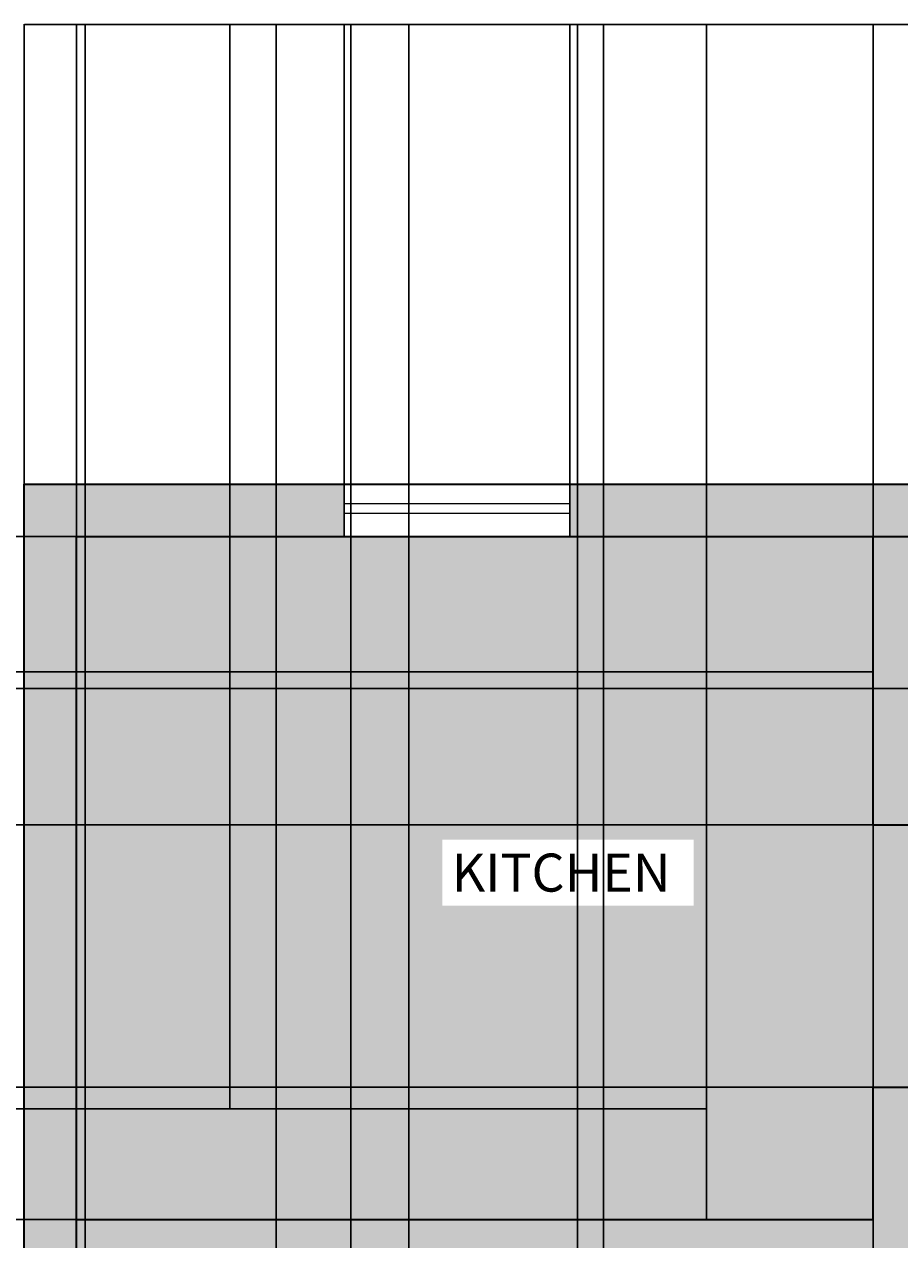
# Model space of a CAD drawing. Units: millimetres. Extents: x -229 to 16545, y -10488 to 4272.
# Tile 5 of 29: x 2016 to 5862, y -1067 to 4272. Entities that reach past the tile are written whole.
import ezdxf

# ---------------------------------------------------------------- set-up
doc = ezdxf.new("R2010")
doc.units = ezdxf.units.MM
for name, color, linetype, lineweight in [('A-ANNO-DIMS', 2, 'Continuous', 18), ('A-AREA-IDEN', 7, 'Continuous', 18), ('A-FLOR-CASE', 7, 'Continuous', 25), ('A-GLAZ', 4, 'Continuous', 18), ('A-WALL', 7, 'Continuous', 35)]:
    doc.layers.add(name, color=color, linetype=linetype, lineweight=lineweight)
for name, color, linetype, lineweight, true_color in [('A-FLOR-CASE-PATT', 252, 'Continuous', 13, 0x939598), ('A-FLOR-PATT', 254, 'Continuous', 13, 0xfeeab9), ('A-WALL-PATT', 18, 'Continuous', 13, 0x000000)]:
    doc.layers.add(name, color=color, linetype=linetype, lineweight=lineweight, true_color=true_color)
doc.styles.get("Standard").update_dxf_attribs({"font": 'arial.ttf'})
doc.dimstyles.get("Standard").update_dxf_attribs({"dimtxt": 0.18, "dimasz": 0.18, "dimexe": 0.18, "dimexo": 0.0625, "dimgap": 0.09, "dimtad": 0, "dimtih": 1, "dimtoh": 1, "dimdec": 4, "dimzin": 0, "dimdsep": 46, "dimtxsty": 'Standard', "dimcen": 0.09, "dimadec": 0, "dimazin": 0, "dimtfac": 1, "dimtdec": 4, "dimtofl": 0, "dimtmove": 0, "dimatfit": 3, "dimfxl": 1, "dimtolj": 1, "dimtzin": 0, "dimarcsym": 0})

# ---------------------------------------------------------------- blocks, each defined once
blk = doc.blocks.new('*D45')
at = {"layer": 'A-ANNO-DIMS', "color": 0, "lineweight": -2, "transparency": 16777216}
for p, q in [((2015.9, 2251.8), (2015.9, 4271.7)), ((2016.1, 4271.5), (8015.5, 4271.5)), ((14015.8, 4271.5), (8016.4, 4271.5)), ((14015.9, 2251.8), (14015.9, 4271.7))]:
    blk.add_line(p, q, dxfattribs=at)
at = {"layer": 'A-ANNO-DIMS', "color": 0, "transparency": 16777216}
for points in [[(2016.1, 4271.5), (2016.1, 4271.4), (2015.9, 4271.5)], [(14015.8, 4271.5), (14015.8, 4271.4), (14015.9, 4271.5)]]:
    blk.add_solid(points, dxfattribs=at)
at = {"layer": 'Defpoints', "color": 0, "transparency": 16777216}
for p in [(14015.9, 4271.5), (2015.9, 2251.7), (14015.9, 2251.7)]:
    blk.add_point(p, dxfattribs=at)
at = {"layer": 'A-ANNO-DIMS', "color": 0, "transparency": 16777216, "insert": (8015.9, 4271.5), "char_height": 0.18, "attachment_point": 5}
blk.add_mtext('\\A1;12000', dxfattribs=at)
blk = doc.blocks.new('*D50')
at = {"layer": 'A-ANNO-DIMS', "color": 0, "lineweight": -2, "transparency": 16777216}
for p, q in [((2245.9, -978.2), (2245.9, 4271.7)), ((2246.1, 4271.5), (3995.6, 4271.5)), ((5745.8, 4271.5), (3996.3, 4271.5)), ((5745.9, -978.2), (5745.9, 4271.7))]:
    blk.add_line(p, q, dxfattribs=at)
at = {"layer": 'A-ANNO-DIMS', "color": 0, "transparency": 16777216}
for points in [[(2246.1, 4271.5), (2246.1, 4271.4), (2245.9, 4271.5)], [(5745.8, 4271.5), (5745.8, 4271.4), (5745.9, 4271.5)]]:
    blk.add_solid(points, dxfattribs=at)
at = {"layer": 'Defpoints', "color": 0, "transparency": 16777216}
for p in [(5745.9, 4271.5), (2245.9, -978.3), (5745.9, -978.3)]:
    blk.add_point(p, dxfattribs=at)
at = {"layer": 'A-ANNO-DIMS', "color": 0, "transparency": 16777216, "insert": (3995.9, 4271.5), "char_height": 0.18, "attachment_point": 5}
blk.add_mtext('\\A1;3500', dxfattribs=at)
blk = doc.blocks.new('*D53')
at = {"layer": 'A-ANNO-DIMS', "color": 0, "lineweight": -2, "transparency": 16777216}
for p, q in [((2245.9, 2021.7), (-228.8, 2021.7)), ((-228.7, 2021.5), (-228.7, 521.9)), ((-228.7, -978.1), (-228.7, 521.5)), ((2245.9, -978.3), (-228.8, -978.3))]:
    blk.add_line(p, q, dxfattribs=at)
at = {"layer": 'A-ANNO-DIMS', "color": 0, "transparency": 16777216}
for points in [[(-228.7, 2021.5), (-228.6, 2021.5), (-228.7, 2021.7)], [(-228.7, -978.1), (-228.6, -978.1), (-228.7, -978.3)]]:
    blk.add_solid(points, dxfattribs=at)
at = {"layer": 'Defpoints', "color": 0, "transparency": 16777216}
for p in [(2245.9, 2021.7), (-228.7, -978.3), (2245.9, -978.3)]:
    blk.add_point(p, dxfattribs=at)
at = {"layer": 'A-ANNO-DIMS', "color": 0, "transparency": 16777216, "insert": (-228.7, 521.7), "char_height": 0.18, "attachment_point": 5}
blk.add_mtext('\\A1;3000', dxfattribs=at)
blk = doc.blocks.new('*D54')
at = {"layer": 'A-ANNO-DIMS', "color": 0, "lineweight": -2, "transparency": 16777216}
for p, q in [((2245.933029, -2708.209552), (2245.933029, 4271.65929)), ((2246.113029, 4271.47929), (3345.573029, 4271.47929)), ((4445.753029, 4271.47929), (3346.293029, 4271.47929)), ((4445.933029, -2708.209552), (4445.933029, 4271.65929))]:
    blk.add_line(p, q, dxfattribs=at)
at = {"layer": 'A-ANNO-DIMS', "color": 0, "transparency": 16777216}
for points in [[(2246.113029, 4271.50929), (2246.113029, 4271.44929), (2245.933029, 4271.47929)], [(4445.753029, 4271.50929), (4445.753029, 4271.44929), (4445.933029, 4271.47929)]]:
    blk.add_solid(points, dxfattribs=at)
at = {"layer": 'Defpoints', "color": 0, "transparency": 16777216}
for p in [(4445.933029, 4271.47929), (2245.933029, -2708.272052), (4445.933029, -2708.272052)]:
    blk.add_point(p, dxfattribs=at)
at = {"layer": 'A-ANNO-DIMS', "color": 0, "transparency": 16777216, "insert": (3345.933029, 4271.47929), "char_height": 0.18, "attachment_point": 5}
blk.add_mtext('\\A1;2200', dxfattribs=at)
blk = doc.blocks.new('*D64')
at = {"layer": 'A-ANNO-DIMS', "color": 0, "lineweight": -2, "transparency": 16777216}
for p, q in [((5745.9, 755.5), (-228.8, 755.5)), ((-228.7, 755.3), (-228.7, 179.2)), ((-228.7, -397.3), (-228.7, 178.8)), ((5745.9, -397.5), (-228.8, -397.5))]:
    blk.add_line(p, q, dxfattribs=at)
at = {"layer": 'A-ANNO-DIMS', "color": 0, "transparency": 16777216}
for points in [[(-228.7, 755.3), (-228.6, 755.3), (-228.7, 755.5)], [(-228.7, -397.3), (-228.6, -397.3), (-228.7, -397.5)]]:
    blk.add_solid(points, dxfattribs=at)
at = {"layer": 'Defpoints', "color": 0, "transparency": 16777216}
for p in [(5745.9, 755.5), (-228.7, -397.5), (5745.9, -397.5)]:
    blk.add_point(p, dxfattribs=at)
at = {"layer": 'A-ANNO-DIMS', "color": 0, "transparency": 16777216, "insert": (-228.7, 179), "char_height": 0.18, "attachment_point": 5}
blk.add_mtext('\\A1;1153', dxfattribs=at)
blk = doc.blocks.new('*D69')
at = {"layer": 'A-ANNO-DIMS', "color": 0, "lineweight": -2, "transparency": 16777216}
for p, q in [((2245.9, 2021.8), (2245.9, 4271.7)), ((2246.1, 4271.5), (2833, 4271.5)), ((3420.7, 4271.5), (2833.7, 4271.5)), ((3420.9, 2021.8), (3420.9, 4271.7))]:
    blk.add_line(p, q, dxfattribs=at)
at = {"layer": 'A-ANNO-DIMS', "color": 0, "transparency": 16777216}
for points in [[(2246.1, 4271.5), (2246.1, 4271.4), (2245.9, 4271.5)], [(3420.7, 4271.5), (3420.7, 4271.4), (3420.9, 4271.5)]]:
    blk.add_solid(points, dxfattribs=at)
at = {"layer": 'Defpoints', "color": 0, "transparency": 16777216}
for p in [(3420.9, 4271.5), (2245.9, 2021.7), (3420.9, 2021.7)]:
    blk.add_point(p, dxfattribs=at)
at = {"layer": 'A-ANNO-DIMS', "color": 0, "transparency": 16777216, "insert": (2833.4, 4271.5), "char_height": 0.18, "attachment_point": 5}
blk.add_mtext('\\A1;1175', dxfattribs=at)
blk = doc.blocks.new('*D70')
at = {"layer": 'A-ANNO-DIMS', "color": 0, "lineweight": -2, "transparency": 16777216}
for p, q in [((3420.9, 2021.8), (3420.9, 4271.7)), ((3421, 4271.5), (3916.4, 4271.5)), ((4412.5, 4271.5), (3917.2, 4271.5)), ((4412.7, 2021.8), (4412.7, 4271.7))]:
    blk.add_line(p, q, dxfattribs=at)
at = {"layer": 'A-ANNO-DIMS', "color": 0, "transparency": 16777216}
for points in [[(3421, 4271.5), (3421, 4271.4), (3420.9, 4271.5)], [(4412.5, 4271.5), (4412.5, 4271.4), (4412.7, 4271.5)]]:
    blk.add_solid(points, dxfattribs=at)
at = {"layer": 'Defpoints', "color": 0, "transparency": 16777216}
for p in [(4412.7, 4271.5), (3420.9, 2021.7), (4412.7, 2021.7)]:
    blk.add_point(p, dxfattribs=at)
at = {"layer": 'A-ANNO-DIMS', "color": 0, "transparency": 16777216, "insert": (3916.8, 4271.5), "char_height": 0.18, "attachment_point": 5}
blk.add_mtext('\\A1;991.9', dxfattribs=at)
blk = doc.blocks.new('*D75')
at = {"layer": 'A-ANNO-DIMS', "color": 0, "lineweight": -2, "transparency": 16777216}
for p, q in [((2245.9, -978.2), (2245.9, 4271.7)), ((2246.1, 4271.5), (2582, 4271.5)), ((2918.6, 4271.5), (2582.8, 4271.5)), ((2918.8, -492.9), (2918.8, 4271.7))]:
    blk.add_line(p, q, dxfattribs=at)
at = {"layer": 'A-ANNO-DIMS', "color": 0, "transparency": 16777216}
for points in [[(2246.1, 4271.5), (2246.1, 4271.4), (2245.9, 4271.5)], [(2918.6, 4271.5), (2918.6, 4271.4), (2918.8, 4271.5)]]:
    blk.add_solid(points, dxfattribs=at)
at = {"layer": 'Defpoints', "color": 0, "transparency": 16777216}
for p in [(2918.8, 4271.5), (2918.8, -492.9), (2245.9, -978.3)]:
    blk.add_point(p, dxfattribs=at)
at = {"layer": 'A-ANNO-DIMS', "color": 0, "transparency": 16777216, "insert": (2582.4, 4271.5), "char_height": 0.18, "attachment_point": 5}
blk.add_mtext('\\A1;672.9', dxfattribs=at)
blk = doc.blocks.new('*D76')
at = {"layer": 'A-ANNO-DIMS', "color": 0, "lineweight": -2, "transparency": 16777216}
for p, q in [((5745.9, 2021.7), (-228.8, 2021.7)), ((-228.7, 2021.5), (-228.7, 1724.7)), ((-228.7, 1427.4), (-228.7, 1724.3)), ((5745.9, 1427.3), (-228.8, 1427.3))]:
    blk.add_line(p, q, dxfattribs=at)
at = {"layer": 'A-ANNO-DIMS', "color": 0, "transparency": 16777216}
for points in [[(-228.7, 2021.5), (-228.6, 2021.5), (-228.7, 2021.7)], [(-228.7, 1427.4), (-228.6, 1427.4), (-228.7, 1427.3)]]:
    blk.add_solid(points, dxfattribs=at)
at = {"layer": 'Defpoints', "color": 0, "transparency": 16777216}
for p in [(5745.9, 2021.7), (-228.7, 1427.3), (5745.9, 1427.3)]:
    blk.add_point(p, dxfattribs=at)
at = {"layer": 'A-ANNO-DIMS', "color": 0, "transparency": 16777216, "insert": (-228.7, 1724.5), "char_height": 0.18, "attachment_point": 5}
blk.add_mtext('\\A1;594.5', dxfattribs=at)
blk = doc.blocks.new('*D77')
at = {"layer": 'A-ANNO-DIMS', "color": 0, "lineweight": -2, "transparency": 16777216}
for p, q in [((2918.8, -492.9), (2918.8, 4271.7)), ((2919, 4271.5), (3965.6, 4271.5)), ((5013.1, 4271.5), (3966.5, 4271.5)), ((5013.3, -492.9), (5013.3, 4271.7))]:
    blk.add_line(p, q, dxfattribs=at)
at = {"layer": 'A-ANNO-DIMS', "color": 0, "transparency": 16777216}
for points in [[(2919, 4271.5), (2919, 4271.4), (2918.8, 4271.5)], [(5013.1, 4271.5), (5013.1, 4271.4), (5013.3, 4271.5)]]:
    blk.add_solid(points, dxfattribs=at)
at = {"layer": 'Defpoints', "color": 0, "transparency": 16777216}
for p in [(5013.3, 4271.5), (2918.8, -492.9), (5013.3, -492.9)]:
    blk.add_point(p, dxfattribs=at)
at = {"layer": 'A-ANNO-DIMS', "color": 0, "transparency": 16777216, "insert": (3966.1, 4271.5), "char_height": 0.18, "attachment_point": 5}
blk.add_mtext('\\A1;2094.5', dxfattribs=at)
blk = doc.blocks.new('*D78')
at = {"layer": 'A-ANNO-DIMS', "color": 0, "lineweight": -2, "transparency": 16777216}
for p, q in [((5013.3, -492.9), (-228.8, -492.9)), ((-228.7, -493.1), (-228.7, -735.4)), ((-228.7, -978.1), (-228.7, -735.8)), ((5013.3, -978.3), (-228.8, -978.3))]:
    blk.add_line(p, q, dxfattribs=at)
at = {"layer": 'A-ANNO-DIMS', "color": 0, "transparency": 16777216}
for points in [[(-228.7, -493.1), (-228.6, -493.1), (-228.7, -492.9)], [(-228.7, -978.1), (-228.6, -978.1), (-228.7, -978.3)]]:
    blk.add_solid(points, dxfattribs=at)
at = {"layer": 'Defpoints', "color": 0, "transparency": 16777216}
for p in [(-228.7, -492.9), (5013.3, -492.9), (5013.3, -978.3)]:
    blk.add_point(p, dxfattribs=at)
at = {"layer": 'A-ANNO-DIMS', "color": 0, "transparency": 16777216, "insert": (-228.7, -735.6), "char_height": 0.18, "attachment_point": 5}
blk.add_mtext('\\A1;485.3', dxfattribs=at)
blk = doc.blocks.new('*D81')
at = {"layer": 'A-ANNO-DIMS', "color": 0, "lineweight": -2, "transparency": 16777216}
for p, q in [((2245.9, -2823.2), (2245.9, 4271.7)), ((2246.1, 4271.5), (2847.7, 4271.5)), ((3450.2, 4271.5), (2848.6, 4271.5)), ((3450.4, -2823.2), (3450.4, 4271.7))]:
    blk.add_line(p, q, dxfattribs=at)
at = {"layer": 'A-ANNO-DIMS', "color": 0, "transparency": 16777216}
for points in [[(2246.1, 4271.5), (2246.1, 4271.4), (2245.9, 4271.5)], [(3450.2, 4271.5), (3450.2, 4271.4), (3450.4, 4271.5)]]:
    blk.add_solid(points, dxfattribs=at)
at = {"layer": 'Defpoints', "color": 0, "transparency": 16777216}
for p in [(3450.4, 4271.5), (2245.9, -2823.3), (3450.4, -2823.3)]:
    blk.add_point(p, dxfattribs=at)
at = {"layer": 'A-ANNO-DIMS', "color": 0, "transparency": 16777216, "insert": (2848.2, 4271.5), "char_height": 0.18, "attachment_point": 5}
blk.add_mtext('\\A1;1204.5', dxfattribs=at)
blk = doc.blocks.new('*D82')
at = {"layer": 'A-ANNO-DIMS', "color": 0, "lineweight": -2, "transparency": 16777216}
for p, q in [((3450.4, -2823.2), (3450.4, 4271.7)), ((3450.6, 4271.5), (3577.5, 4271.5)), ((3705.3, 4271.5), (3578.4, 4271.5)), ((3705.5, -2823.2), (3705.5, 4271.7))]:
    blk.add_line(p, q, dxfattribs=at)
at = {"layer": 'A-ANNO-DIMS', "color": 0, "transparency": 16777216}
for points in [[(3450.6, 4271.5), (3450.6, 4271.4), (3450.4, 4271.5)], [(3705.3, 4271.5), (3705.3, 4271.4), (3705.5, 4271.5)]]:
    blk.add_solid(points, dxfattribs=at)
at = {"layer": 'Defpoints', "color": 0, "transparency": 16777216}
for p in [(3705.5, 4271.5), (3450.4, -2823.3), (3705.5, -2823.3)]:
    blk.add_point(p, dxfattribs=at)
at = {"layer": 'A-ANNO-DIMS', "color": 0, "transparency": 16777216, "insert": (3577.9, 4271.5), "char_height": 0.18, "attachment_point": 5}
blk.add_mtext('\\A1;255.06', dxfattribs=at)
blk = doc.blocks.new('*D84')
at = {"layer": 'A-ANNO-DIMS', "color": 0, "lineweight": -2, "transparency": 16777216}
for p, q in [((4445.9, -2708.2), (4445.9, 4271.7)), ((4446.1, 4271.5), (4503.2, 4271.5)), ((4560.8, 4271.5), (4503.7, 4271.5)), ((4560.9, -2823.2), (4560.9, 4271.7))]:
    blk.add_line(p, q, dxfattribs=at)
at = {"layer": 'A-ANNO-DIMS', "color": 0, "transparency": 16777216}
for points in [[(4446.1, 4271.5), (4446.1, 4271.4), (4445.9, 4271.5)], [(4560.8, 4271.5), (4560.8, 4271.4), (4560.9, 4271.5)]]:
    blk.add_solid(points, dxfattribs=at)
at = {"layer": 'Defpoints', "color": 0, "transparency": 16777216}
for p in [(4560.9, 4271.5), (4445.9, -2708.3), (4560.9, -2823.3)]:
    blk.add_point(p, dxfattribs=at)
at = {"layer": 'A-ANNO-DIMS', "color": 0, "transparency": 16777216, "insert": (4503.4, 4271.5), "char_height": 0.18, "attachment_point": 5}
blk.add_mtext('\\A1;115', dxfattribs=at)
blk = doc.blocks.new('*D85')
at = {"layer": 'A-ANNO-DIMS', "color": 0, "lineweight": -2, "transparency": 16777216}
for p, q in [((5745.9, 755.6), (5745.9, 4271.7)), ((5746.1, 4271.5), (5860.6, 4271.5)), ((5975.8, 4271.5), (5861.2, 4271.5)), ((5975.9, 755.6), (5975.9, 4271.7))]:
    blk.add_line(p, q, dxfattribs=at)
at = {"layer": 'A-ANNO-DIMS', "color": 0, "transparency": 16777216}
for points in [[(5746.1, 4271.5), (5746.1, 4271.4), (5745.9, 4271.5)], [(5975.8, 4271.5), (5975.8, 4271.4), (5975.9, 4271.5)]]:
    blk.add_solid(points, dxfattribs=at)
at = {"layer": 'Defpoints', "color": 0, "transparency": 16777216}
for p in [(5975.9, 4271.5), (5745.9, 755.5), (5975.9, 755.5)]:
    blk.add_point(p, dxfattribs=at)
at = {"layer": 'A-ANNO-DIMS', "color": 0, "transparency": 16777216, "insert": (5860.9, 4271.5), "char_height": 0.18, "attachment_point": 5}
blk.add_mtext('\\A1;230', dxfattribs=at)
blk = doc.blocks.new('*D89')
at = {"layer": 'A-ANNO-DIMS', "color": 0, "lineweight": -2, "transparency": 16777216}
for p, q in [((5745.9, -397.5), (-228.8, -397.5)), ((-228.7, -397.7), (-228.7, -687.7)), ((-228.7, -978.1), (-228.7, -688.1)), ((5745.9, -978.3), (-228.8, -978.3))]:
    blk.add_line(p, q, dxfattribs=at)
at = {"layer": 'A-ANNO-DIMS', "color": 0, "transparency": 16777216}
for points in [[(-228.7, -397.7), (-228.6, -397.7), (-228.7, -397.5)], [(-228.7, -978.1), (-228.6, -978.1), (-228.7, -978.3)]]:
    blk.add_solid(points, dxfattribs=at)
at = {"layer": 'Defpoints', "color": 0, "transparency": 16777216}
for p in [(5745.9, -397.5), (-228.7, -978.3), (5745.9, -978.3)]:
    blk.add_point(p, dxfattribs=at)
at = {"layer": 'A-ANNO-DIMS', "color": 0, "transparency": 16777216, "insert": (-228.7, -687.9), "char_height": 0.18, "attachment_point": 5}
blk.add_mtext('\\A1;580.8', dxfattribs=at)
blk = doc.blocks.new('*D93')
at = {"layer": 'A-ANNO-DIMS', "color": 0, "lineweight": -2, "transparency": 16777216}
for p, q in [((2284, -1683.4), (2284, 4271.7)), ((2284.2, 4271.5), (2702.7, 4271.5)), ((3122, 4271.5), (2703.5, 4271.5)), ((3122.2, -1950.1), (3122.2, 4271.7))]:
    blk.add_line(p, q, dxfattribs=at)
at = {"layer": 'A-ANNO-DIMS', "color": 0, "transparency": 16777216}
for points in [[(2284.2, 4271.5), (2284.2, 4271.4), (2284, 4271.5)], [(3122, 4271.5), (3122, 4271.4), (3122.2, 4271.5)]]:
    blk.add_solid(points, dxfattribs=at)
at = {"layer": 'Defpoints', "color": 0, "transparency": 16777216}
for p in [(3122.2, 4271.5), (2284, -1683.5), (3122.2, -1950.2)]:
    blk.add_point(p, dxfattribs=at)
at = {"layer": 'A-ANNO-DIMS', "color": 0, "transparency": 16777216, "insert": (2703.1, 4271.5), "char_height": 0.18, "attachment_point": 5}
blk.add_mtext('\\A1;838.2', dxfattribs=at)
blk = doc.blocks.new('*D97')
at = {"layer": 'A-ANNO-DIMS', "color": 0, "lineweight": -2, "transparency": 16777216}
for p, q in [((3450.4, -2823.2), (3450.4, 4271.7)), ((3450.6, 4271.5), (4597.7, 4271.5)), ((5745.8, 4271.5), (4598.6, 4271.5)), ((5745.9, -2823.2), (5745.9, 4271.7))]:
    blk.add_line(p, q, dxfattribs=at)
at = {"layer": 'A-ANNO-DIMS', "color": 0, "transparency": 16777216}
for points in [[(3450.6, 4271.5), (3450.6, 4271.4), (3450.4, 4271.5)], [(5745.8, 4271.5), (5745.8, 4271.4), (5745.9, 4271.5)]]:
    blk.add_solid(points, dxfattribs=at)
at = {"layer": 'Defpoints', "color": 0, "transparency": 16777216}
for p in [(5745.9, 4271.5), (3450.4, -2823.3), (5745.9, -2823.3)]:
    blk.add_point(p, dxfattribs=at)
at = {"layer": 'A-ANNO-DIMS', "color": 0, "transparency": 16777216, "insert": (4598.2, 4271.5), "char_height": 0.18, "attachment_point": 5}
blk.add_mtext('\\A1;2295.5', dxfattribs=at)
blk = doc.blocks.new('*D100')
at = {"layer": 'A-ANNO-DIMS', "color": 0, "lineweight": -2, "transparency": 16777216}
for p, q in [((7294.4, 2021.7), (-228.8, 2021.7)), ((-228.7, 2021.5), (-228.7, 1688.2)), ((-228.7, 1354.6), (-228.7, 1687.9)), ((8024.8, 1354.4), (-228.8, 1354.4))]:
    blk.add_line(p, q, dxfattribs=at)
at = {"layer": 'A-ANNO-DIMS', "color": 0, "transparency": 16777216}
for points in [[(-228.7, 2021.5), (-228.6, 2021.5), (-228.7, 2021.7)], [(-228.7, 1354.6), (-228.6, 1354.6), (-228.7, 1354.4)]]:
    blk.add_solid(points, dxfattribs=at)
at = {"layer": 'Defpoints', "color": 0, "transparency": 16777216}
for p in [(7294.4, 2021.7), (-228.7, 1354.4), (8024.9, 1354.4)]:
    blk.add_point(p, dxfattribs=at)
at = {"layer": 'A-ANNO-DIMS', "color": 0, "transparency": 16777216, "insert": (-228.7, 1688.1), "char_height": 0.18, "attachment_point": 5}
blk.add_mtext('\\A1;667.3', dxfattribs=at)

msp = doc.modelspace()

# ---------------------------------------------------------------- hatches: boundary and pattern name
at = {"layer": 'A-FLOR-CASE-PATT', "transparency": 33554646}
h = msp.add_hatch(color=256, dxfattribs=at)
h.dxf.hatch_style = 1
h.paths.add_polyline_path([(2918.813, 1427.266), (5745.933, 1427.266), (5745.933, 2021.728), (2245.933, 2021.728), (2245.933, -978.272), (5013.319, -978.272), (5013.319, -492.942), (2918.813, -492.942)])
at = {"layer": 'A-FLOR-PATT', "transparency": 33554592}
h = msp.add_hatch(color=256, dxfattribs=at)
h.dxf.hatch_style = 1
h.paths.add_polyline_path([(7975.933, -5325.772), (7943.121, -5325.772), (7943.121, -4576.49, 0.40145271), (7225.933, -5325.772, 0.40145271), (6508.746, -4576.49), (6508.746, -5325.772), (6475.933, -5325.772), (6475.933, -5438.272), (5975.933, -5438.272), (5975.933, -7267.724), (5975.933, -7438.272), (6478.619, -7438.272), (6463.448, -7355.919), (6464.88, -7356.837), (6463.849, -7358.097), (6478.619, -7438.272), (6610.327, -7438.272), (6632.656, -7409.564), (6632.525, -7406.967), (6634.208, -7407.569), (6619.273, -7426.77), (6654.466, -7438.272), (7610.517, -7438.272), (7607.41, -7421.409), (7608.842, -7422.327), (7607.812, -7423.587), (7610.517, -7438.272), (7975.933, -7438.272)])
h.paths.add_polyline_path([(13785.933, -1208.272), (9555.933, -1208.272), (9555.933, -961.785), (9705.933, -961.785), (9705.933, -918.035), (10704.976, -918.035, 0.40145271), (9705.933, 38.215), (9555.933, 38.215), (9555.933, 2021.728), (5975.933, 2021.728), (5975.933, 755.492), (5745.933, 755.492), (5745.933, 1427.266), (2918.813, 1427.266), (2918.813, -492.942), (5013.319, -492.942), (5013.319, -978.272), (5745.933, -978.272), (5745.933, -397.513), (5975.933, -397.513), (5975.933, -1208.272), (4560.933, -1208.272), (4560.933, -1265.772), (4448.433, -1265.772), (4448.433, -1298.585), (4445.933, -1298.585), (3699.151, -1298.585, 0.40145271), (4448.433, -2015.772), (4560.933, -2015.772), (4560.933, -2384.177), (5745.933, -2384.177), (5799.402, -2384.177), (5799.402, -4518.272), (5975.933, -4518.272), (5975.933, -5208.272), (6475.933, -5208.272), (6475.933, -4575.772), (6508.746, -4575.772), (6508.746, -4576.49, -0.35647263), (7216.672, -5208.272), (7235.194, -5208.272, -0.35647263), (7943.121, -4576.49), (7943.121, -4575.772), (7975.933, -4575.772), (7975.933, -5208.272), (11176.247, -5208.272), (11159.44, -5191.465), (10520.768, -5191.465), (10520.768, -4888.936), (10571.19, -4888.936), (10571.19, -4872.129), (10772.876, -4872.129), (10772.876, -4888.936), (10789.683, -4888.936), (10789.683, -4872.129), (10991.368, -4872.129), (10991.368, -4888.936), (11041.79, -4888.936), (11041.79, -4872.129), (11058.597, -4872.129, -0.09090909), (11428.354, -4872.129), (11445.162, -4872.129), (11445.162, -4888.936), (11529.197, -4888.936), (11529.197, -5191.465), (11327.512, -5191.465), (11310.704, -5208.272), (13785.933, -5208.272)])
h.paths.add_polyline_path([(11047.216, -1630.944, -1), (11402.816, -1630.944, -1)], flags=16)
h.paths.add_polyline_path([(11148.816, -1630.944), (11225.016, -1554.744), (11301.216, -1630.944), (11225.016, -1707.144)], flags=0)
h.paths.add_polyline_path([(11199.616, -1630.944, -1), (11250.416, -1630.944, -1)], flags=0)
h.paths.add_polyline_path([(11588.751, -2096.259), (11588.751, -1543.254, -0.26666697), (12864.918, -1543.254), (12864.918, -2096.259), (12737.302, -2096.259), (12737.302, -2063.121), (11716.368, -2063.121), (11716.368, -2096.259)], flags=16)
h.paths.add_polyline_path([(12012.696, -2489.42), (12600.997, -2489.42), (12600.997, -3666.022), (12012.696, -3666.022)], flags=16)
h.paths.add_polyline_path([(12176.41, -3599.403), (12174.938, -3609.076), (12173.789, -3618.819), (12173.09, -3628.559), (12172.973, -3638.221), (12173.89, -3652.852), (12175.008, -3657.025), (12172.909, -3643.473), (12173.142, -3624.297), (12175.386, -3605.273)], flags=0)
h.paths.add_polyline_path([(8026.289, -286.944), (7737.703, -287.19), (7734.87, -269.156), (8029.092, -268.905)], flags=16)
h.paths.add_polyline_path([(7733.453, -260.139), (7710.784, -115.865), (7557.191, -115.996), (7556.999, 109.744), (7412.687, 132.166), (7412.433, 429.206), (7556.707, 451.876), (7556.568, 614.769), (7412.256, 637.19), (7412.003, 934.231), (7556.276, 956.9), (7556.084, 1182.639), (7709.677, 1182.77), (7732.099, 1327.082), (8029.14, 1327.335), (8051.808, 1183.062), (8205.401, 1183.192), (8205.594, 957.454), (8349.906, 935.031), (8350.159, 637.99), (8205.885, 615.322), (8206.024, 452.43), (8350.336, 430.006), (8350.59, 132.965), (8206.316, 110.298), (8206.509, -115.442), (8052.916, -115.573), (8030.493, -259.885)], flags=16)
h.paths.add_polyline_path([(12261.416, -3475.554), (12262.632, -3486.776), (12264.032, -3497.007), (12265.554, -3506.365), (12267.136, -3514.968), (12268.719, -3522.935), (12271.304, -3535.59), (12273.606, -3548.078), (12275.271, -3561.064), (12275.93, -3574.938), (12275.325, -3590.3), (12273.425, -3607.964), (12270.795, -3625.658), (12268.066, -3641.063), (12266.318, -3649.679), (12265.456, -3653.626), (12263.984, -3659.846), (12264.032, -3659.566), (12264.342, -3658.241), (12264.807, -3656.37), (12265.456, -3653.626), (12266.318, -3649.679), (12267.409, -3644.302), (12268.668, -3637.664), (12270.019, -3630.037), (12271.384, -3621.695), (12272.69, -3612.908), (12273.857, -3603.948), (12274.81, -3595.088), (12275.47, -3586.601), (12275.782, -3578.689), (12275.757, -3571.292), (12275.423, -3564.275), (12274.816, -3557.512), (12273.964, -3550.872), (12272.896, -3544.224), (12271.645, -3537.439), (12270.24, -3530.385), (12267.543, -3517.181), (12264.612, -3501.247), (12261.849, -3481.059)], flags=0)
h.paths.add_polyline_path([(12332.136, -3408.03), (12333.483, -3416.79), (12335.077, -3424.54), (12336.915, -3431.355), (12338.991, -3437.32), (12341.266, -3442.55), (12343.694, -3447.166), (12346.229, -3451.292), (12348.826, -3455.051), (12351.438, -3458.563), (12357.476, -3466.491), (12363.61, -3476.575), (12368.309, -3489.762), (12369.929, -3503.427), (12369.842, -3516.511), (12368.43, -3530.867), (12365.816, -3545.835), (12362.382, -3559.786), (12360.968, -3564.487), (12363.063, -3557.021), (12364.898, -3549.566), (12366.473, -3542.077), (12367.773, -3534.631), (12368.781, -3527.301), (12369.483, -3520.162), (12369.863, -3513.291), (12369.906, -3506.759), (12369.599, -3500.643), (12368.93, -3494.999), (12367.924, -3489.796), (12366.61, -3484.994), (12365.024, -3480.542), (12363.19, -3476.399), (12361.141, -3472.516), (12358.909, -3468.847), (12356.525, -3465.347), (12354.02, -3461.954), (12351.438, -3458.563), (12345.462, -3450.529), (12339.923, -3439.996), (12335.85, -3428.296), (12332.68, -3412.888)], flags=0)
h.paths.add_polyline_path([(12385.287, -3334.612), (12384.977, -3342.409), (12385.02, -3349.196), (12385.4, -3355.066), (12386.104, -3360.105), (12387.112, -3364.41), (12388.412, -3368.071), (12389.987, -3371.181), (12391.823, -3373.832), (12393.919, -3376.097), (12396.337, -3377.978), (12399.153, -3379.462), (12402.445, -3380.531), (12406.289, -3381.172), (12410.758, -3381.371), (12415.935, -3381.106), (12421.893, -3380.368), (12428.658, -3379.159), (12436.069, -3377.55), (12443.907, -3375.635), (12451.961, -3373.505), (12460.015, -3371.254), (12467.853, -3368.971), (12475.263, -3366.749), (12482.029, -3364.68), (12491.877, -3361.657), (12497.701, -3360.107), (12501.639, -3359.288), (12510.135, -3358.326), (12519.662, -3365.412), (12524.243, -3378.911), (12523.764, -3390.7), (12520.746, -3401.577), (12514.248, -3415.634), (12511.518, -3420.418), (12515.856, -3412.154), (12519.153, -3405.024), (12521.516, -3398.804), (12523.049, -3393.276), (12523.865, -3388.212), (12524.059, -3383.441), (12523.7, -3378.958), (12522.853, -3374.815), (12521.576, -3371.054), (12519.931, -3367.722), (12517.982, -3364.865), (12515.786, -3362.529), (12513.405, -3360.758), (12510.877, -3359.588), (12508.136, -3358.982), (12505.086, -3358.897), (12501.639, -3359.288), (12497.701, -3360.107), (12493.183, -3361.309), (12487.988, -3362.851), (12476.403, -3366.408), (12463.335, -3370.326), (12447.372, -3374.788), (12431.759, -3378.604), (12418.504, -3380.974), (12405.811, -3381.624), (12394.725, -3378.025), (12388.039, -3368.367), (12385.583, -3357.877), (12384.826, -3346.204), (12385.428, -3331.059), (12385.953, -3325.719)], flags=0)
h.paths.add_polyline_path([(7880.016, 1173.969), (7880.373, 1175.495), (7880.433, 1175.851), (7879.484, 1171.818)], flags=0)
h.paths.add_polyline_path([(7802.33, 874.962), (7800.771, 885.032), (7798.932, 893.941), (7796.811, 901.774), (7794.419, 908.63), (7791.798, 914.639), (7789.002, 919.945), (7786.083, 924.686), (7783.093, 929.005), (7780.087, 933.043), (7774.996, 939.717), (7768.406, 949.37), (7762.174, 963.427), (7759.342, 978.002), (7758.629, 991.888), (7759.492, 1007.928), (7761.801, 1025.496), (7765.392, 1044.035), (7766.625, 1049.048), (7764.522, 1039.543), (7762.719, 1030.232), (7761.232, 1021.168), (7760.08, 1012.405), (7759.28, 1003.994), (7758.849, 995.988), (7758.806, 988.44), (7759.167, 981.404), (7759.942, 974.914), (7761.104, 968.936), (7762.617, 963.414), (7764.448, 958.299), (7766.559, 953.535), (7768.918, 949.073), (7771.487, 944.856), (7774.232, 940.835), (7777.115, 936.938), (7782.377, 930.041), (7787.845, 922.139), (7793.348, 911.698), (7798.042, 898.247), (7801.702, 880.527)], flags=0)
h.paths.add_polyline_path([(12519.068, -3228.534), (12519.615, -3236.235), (12520.529, -3242.343), (12521.78, -3247.103), (12523.337, -3250.758), (12525.171, -3253.556), (12527.248, -3255.709), (12529.522, -3257.296), (12531.95, -3258.361), (12534.486, -3258.949), (12537.082, -3259.11), (12539.694, -3258.888), (12542.277, -3258.329), (12544.781, -3257.478), (12547.173, -3256.388), (12549.46, -3255.129), (12550.455, -3254.517), (12555.825, -3251.109), (12557.835, -3249.942), (12565.181, -3246.404), (12574.565, -3253.032), (12576.931, -3265.022), (12576.627, -3277.425), (12575.416, -3290.819), (12574.851, -3295.392), (12575.708, -3287.593), (12576.322, -3280.806), (12576.688, -3274.939), (12576.812, -3269.899), (12576.688, -3265.593), (12576.322, -3261.932), (12575.708, -3258.822), (12574.851, -3256.172), (12573.753, -3253.905), (12572.439, -3252.005), (12570.943, -3250.474), (12569.293, -3249.309), (12567.523, -3248.513), (12565.658, -3248.083), (12563.732, -3248.022), (12561.777, -3248.328), (12559.814, -3248.989), (12557.835, -3249.942), (12555.825, -3251.109), (12553.77, -3252.413), (12551.652, -3253.78), (12549.46, -3255.129), (12543.167, -3258.594), (12532.661, -3259.485), (12524.685, -3253.923), (12520.949, -3245.152), (12519.138, -3233.042)], flags=0)
h.paths.add_polyline_path([(7741.293, 790.501), (7741.641, 799.467), (7741.584, 807.269), (7741.141, 814.015), (7740.329, 819.809), (7739.165, 824.757), (7737.667, 828.966), (7735.853, 832.541), (7733.74, 835.586), (7731.348, 838.188), (7728.71, 840.348), (7725.861, 842.052), (7722.836, 843.28), (7719.671, 844.015), (7716.4, 844.237), (7713.06, 843.932), (7709.684, 843.081), (7706.304, 841.686), (7702.923, 839.834), (7699.543, 837.629), (7696.164, 835.178), (7692.784, 832.585), (7684.718, 826.315), (7675.609, 820.63), (7664.001, 817.274), (7654.105, 821.884), (7647.171, 832.02), (7644.191, 846.522), (7646.321, 860.288), (7647.49, 864.223), (7645.946, 857.865), (7645.046, 852.044), (7644.827, 846.557), (7645.243, 841.404), (7646.221, 836.642), (7647.693, 832.318), (7649.587, 828.489), (7651.832, 825.206), (7654.359, 822.523), (7657.097, 820.49), (7659.984, 819.145), (7662.993, 818.452), (7666.108, 818.357), (7669.311, 818.809), (7672.583, 819.755), (7675.908, 821.139), (7679.268, 822.913), (7682.645, 825.021), (7686.025, 827.401), (7689.404, 829.958), (7692.784, 832.585), (7700.505, 838.509), (7709.871, 843.64), (7721.436, 844.698), (7733.277, 837.617), (7739.571, 825.214), (7741.557, 811.049), (7741.669, 795.575)], flags=0)
h.paths.add_polyline_path([(8377.641, 137.216), (8359.607, 134.382), (8359.356, 428.605), (8377.395, 425.802)], flags=16)
h.paths.add_polyline_path([(7650.715, 668.465), (7650.08, 677.319), (7649.023, 684.34), (7647.579, 689.811), (7645.785, 694.012), (7643.675, 697.228), (7641.286, 699.7), (7638.669, 701.521), (7635.876, 702.744), (7632.96, 703.419), (7629.974, 703.601), (7626.971, 703.344), (7624.004, 702.697), (7621.125, 701.717), (7618.375, 700.462), (7615.749, 699.013), (7614.561, 698.279), (7608.435, 694.382), (7606.125, 693.04), (7598.981, 689.594), (7589.669, 693.773), (7585.26, 702.856), (7584.221, 713.11), (7584.49, 724.584), (7585.863, 739.937), (7586.518, 745.277), (7585.539, 736.31), (7584.841, 728.507), (7584.424, 721.761), (7584.288, 715.966), (7584.433, 711.016), (7584.86, 706.807), (7585.567, 703.231), (7586.556, 700.186), (7587.821, 697.58), (7589.332, 695.397), (7591.053, 693.637), (7592.951, 692.3), (7594.989, 691.385), (7597.132, 690.895), (7599.346, 690.826), (7601.594, 691.18), (7603.851, 691.943), (7606.125, 693.04), (7608.435, 694.382), (7610.797, 695.885), (7613.229, 697.458), (7620.475, 701.929), (7632.001, 704.44), (7643.476, 699.417), (7648.536, 687.571), (7650.63, 673.661)], flags=0)
h.paths.add_polyline_path([(7385.628, 136.37), (7385.382, 424.956), (7403.416, 427.789), (7403.667, 133.567)], flags=16)
h.paths.add_polyline_path([(12993.884, -2257.186), (12959.588, -2257.186), (12959.588, -2125.099), (13531.966, -2125.099, -0.19047621), (13531.966, -3974.321), (12959.588, -3974.321), (12959.588, -3842.233), (12993.884, -3842.233)], flags=16)
h.paths.add_polyline_path([(13413.486, -3313.884), (13413.486, -2785.535), (13562.885, -2785.535, -0.04962821), (13562.885, -3313.884)], flags=0)
h.paths.add_polyline_path([(8377.21, 642.241), (8359.176, 639.407), (8358.925, 933.629), (8376.964, 930.826)], flags=16)
h.paths.add_polyline_path([(13086.058, -1864.83), (13086.058, -1449.84), (13501.048, -1449.84), (13501.048, -1864.83)], flags=16)
h.paths.add_polyline_path([(13305.814, -1862.197), (13302.103, -1859.624), (13298.088, -1857.068), (13293.799, -1854.536), (13289.262, -1852.031), (13284.504, -1849.559), (13279.554, -1847.125), (13274.439, -1844.735), (13269.17, -1842.389), (13263.701, -1840.081), (13257.97, -1837.797), (13251.914, -1835.525), (13245.472, -1833.252), (13238.582, -1830.968), (13231.18, -1828.66), (13223.206, -1826.315), (13209.182, -1822.458), (13204.584, -1821.48), (13217.962, -1824.773), (13235.072, -1829.804), (13248.777, -1834.349), (13260.829, -1838.869), (13274.479, -1844.63), (13289.675, -1852.101), (13302.553, -1859.704)], flags=0)
h.paths.add_polyline_path([(13428.104, -1820.994), (13419.007, -1818.141), (13409.95, -1815.4), (13400.766, -1812.747), (13391.271, -1810.151), (13376.087, -1806.251), (13370.618, -1805.019), (13386.304, -1808.794), (13405.087, -1813.928), (13423.014, -1819.354)], flags=0)
h.paths.add_polyline_path([(7385.197, 641.395), (7384.951, 929.98), (7402.986, 932.814), (7403.236, 638.592)], flags=16)
h.paths.add_polyline_path([(13262.537, -1725.526), (13253.246, -1724.74), (13244.516, -1724.117), (13235.94, -1723.625), (13223.267, -1723.062), (13217.598, -1722.912), (13231.966, -1723.397), (13248.733, -1724.359), (13266.899, -1725.895), (13272.802, -1726.502)], flags=0)
h.paths.add_polyline_path([(13191.893, -1641.137), (13208.675, -1640.506), (13214.057, -1640.258), (13197.763, -1640.936)], flags=0)
h.paths.add_polyline_path([(13097.524, -1608.457), (13114.284, -1609.031), (13120.126, -1609.105), (13103.045, -1608.71)], flags=0)
h.paths.add_polyline_path([(13465.328, -1521.577), (13473.906, -1517.015), (13481.761, -1511.636), (13492.562, -1502.076), (13495.327, -1497.933), (13485.818, -1508.858), (13470.208, -1519.547)], flags=0)
h.paths.add_polyline_path([(13175.015, -1500.891), (13184.046, -1501.807), (13192.721, -1502.52), (13201.114, -1503.034), (13209.273, -1503.351), (13217.244, -1503.476), (13225.078, -1503.41), (13232.821, -1503.16), (13240.524, -1502.728), (13248.233, -1502.117), (13255.993, -1501.322), (13263.825, -1500.293), (13271.746, -1498.974), (13279.775, -1497.305), (13287.928, -1495.229), (13296.222, -1492.688), (13304.675, -1489.622), (13313.304, -1485.975), (13322.089, -1481.727), (13330.859, -1477.028), (13339.408, -1472.063), (13347.526, -1467.02), (13355.006, -1462.087), (13364.86, -1455.202), (13367.224, -1453.299), (13358.544, -1459.754), (13343.348, -1469.775), (13326.143, -1479.767), (13309.023, -1488.045), (13292.249, -1494.129), (13276.009, -1498.264), (13260.299, -1500.88), (13244.401, -1502.51), (13228.945, -1503.378), (13213.316, -1503.508), (13197.047, -1502.876), (13180.088, -1501.481)], flags=0)
h.paths.add_polyline_path([(7733.501, 1336.101), (7736.303, 1354.14), (8024.889, 1354.386), (8027.723, 1336.352)], flags=16)
at = {"layer": 'A-WALL-PATT'}
h = msp.add_hatch(color=256, dxfattribs=at)
h.dxf.hatch_style = 1
h.paths.add_polyline_path([(7294.425, 2163.983), (7294.425, 2251.728), (4412.722, 2251.728), (4412.722, 2166.741), (4412.722, 2122.457), (4412.722, 2021.728), (7294.425, 2021.728), (7294.425, 2119.698)])
h.paths.add_polyline_path([(11407.51, 2166.741), (11407.51, 2251.728), (8296.763, 2251.728), (8296.763, 2163.983), (8296.763, 2119.698), (8296.763, 2021.728), (11407.51, 2021.728), (11407.51, 2122.457)])
h.paths.add_polyline_path([(9785.933, 2021.728), (9555.933, 2021.728), (9555.933, 38.215), (9705.933, 38.215, -0.02002407), (9785.933, 35.01)])
h.paths.add_polyline_path([(14015.933, 2251.728), (12488.002, 2251.728), (12488.002, 2166.742), (12488.002, 2122.738), (12488.002, 2021.728), (13785.933, 2021.728), (13785.933, -2305.465), (13883.903, -2305.465), (13928.188, -2305.465), (14015.933, -2305.465)])
h.paths.add_polyline_path([(13785.933, -978.272), (9785.933, -978.272), (9785.933, -961.785), (9705.933, -961.785), (9555.933, -961.785), (9555.933, -1208.272), (13785.933, -1208.272)])
h.paths.add_polyline_path([(5975.933, 2021.728), (5745.933, 2021.728), (5745.933, 755.492), (5975.933, 755.492)])
h.paths.add_polyline_path([(2245.933, 2021.728), (3420.865, 2021.728), (3420.865, 2122.457), (3420.865, 2167.104), (3420.865, 2251.728), (2015.933, 2251.728), (2015.933, -3326.811), (2100.943, -3326.811), (2155.199, -3326.811), (2245.933, -3326.811)])
h.paths.add_polyline_path([(5975.933, -397.513), (5745.933, -397.513), (5745.933, -978.272), (2245.933, -978.272), (2245.933, -1208.272), (5975.933, -1208.272)])
h.paths.add_polyline_path([(12015.17, -5208.272), (7975.933, -5208.272), (7975.933, -5325.772), (7975.933, -5438.272), (7975.933, -5596.884), (8205.933, -5596.884), (8205.933, -5438.272), (12015.17, -5438.272), (12015.17, -5337.543), (12015.17, -5293.259)])
h.paths.add_polyline_path([(5975.933, -4518.272), (4567.83, -4518.272), (4567.83, -4603.259), (4567.83, -4647.543), (4567.83, -4748.272), (5745.933, -4748.272), (5745.933, -5438.272), (5975.933, -5438.272), (6475.933, -5438.272), (6475.933, -5325.772), (6475.933, -5208.272), (5975.933, -5208.272)])
h.paths.add_polyline_path([(3765.491, -4518.272), (2245.933, -4518.272), (2245.933, -4748.272), (3765.491, -4748.272), (3765.491, -4647.543), (3765.491, -4603.259)])

# ---------------------------------------------------------------- linework, layer by layer
at = {"layer": 'A-FLOR-CASE', "transparency": 33554569}
for p, q in [((5745.933, 1427.266), (2918.813, 1427.266)), ((2918.813, 1427.266), (2918.813, -492.942)), ((2918.813, -492.942), (5013.319, -492.942)), ((5013.319, -492.942), (5013.319, -978.272))]:
    msp.add_line(p, q, dxfattribs=at)
at = {"layer": 'A-GLAZ'}
for p, q in [((3420.865, 2166.741), (3420.865, 2251.728)), ((4412.722, 2166.741), (4412.722, 2251.728)), ((3420.865, 2122.457), (3420.865, 2021.728)), ((4412.722, 2122.457), (4412.722, 2021.728))]:
    msp.add_line(p, q, dxfattribs=at)
msp.add_lwpolyline([(3420.865, 2167.104), (4412.722, 2166.741), (4412.722, 2122.457), (3420.865, 2122.82)], close=True, dxfattribs=at)
at = {"layer": 'A-WALL'}
for p, q in [((2015.933, 2251.728), (14015.933, 2251.728)), ((2015.933, -9248.272), (2015.933, 2251.728)), ((2245.933, 2021.728), (13785.933, 2021.728)), ((2245.933, -5217.291), (2245.933, 2021.728)), ((5745.933, 755.492), (5745.933, 2021.728)), ((5745.933, 755.492), (5975.933, 755.492)), ((5745.933, -978.272), (5745.933, -397.513)), ((5745.933, -397.513), (5975.933, -397.513)), ((2245.933, -978.272), (5745.933, -978.272))]:
    msp.add_line(p, q, dxfattribs=at)

# ---------------------------------------------------------------- dimensions: what is measured, and where the dimension line sits
at = {"layer": 'A-ANNO-DIMS'}
for base, p1, p2, override, picture, middle in [((14015.933, 4271.479), (2015.933, 2251.728), (14015.933, 2251.728), {"dimdec": 0, "dimlfac": 1, "dimrnd": 0, "dimzin": 0, "dimdsep": 46, "dimlunit": 2}, '*D45', (8015.933, 4271.479)), ((3420.865, 4271.479), (2245.933, 2021.728), (3420.865, 2021.728), {"dimdec": 0, "dimlfac": 1, "dimrnd": 0, "dimzin": 0, "dimdsep": 46, "dimlunit": 2}, '*D69', (2833.399, 4271.479)), ((2918.813, 4271.479), (2245.933, -978.272), (2918.813, -492.942), {"dimdec": 1, "dimlfac": 1, "dimrnd": 0, "dimzin": 0, "dimdsep": 46, "dimlunit": 2}, '*D75', (2582.373, 4271.479)), ((3450.417, 4271.479), (2245.933, -2823.272), (3450.417, -2823.272), {"dimdec": 1, "dimlfac": 1, "dimrnd": 0, "dimzin": 0, "dimdsep": 46, "dimlunit": 2}, '*D81', (2848.175, 4271.479)), ((3122.201, 4271.479), (2284.002, -1683.499), (3122.201, -1950.199), {"dimdec": 1, "dimlfac": 1, "dimrnd": 0, "dimzin": 0, "dimdsep": 46, "dimlunit": 2}, '*D93', (2703.101, 4271.479)), ((4412.722, 4271.479), (3420.865, 2021.728), (4412.722, 2021.728), {"dimdec": 1, "dimlfac": 1, "dimrnd": 0, "dimzin": 0, "dimdsep": 46, "dimlunit": 2}, '*D70', (3916.793, 4271.479)), ((3705.475, 4271.479), (3450.417, -2823.272), (3705.475, -2823.272), {"dimdec": 2, "dimlfac": 1, "dimrnd": 0, "dimzin": 0, "dimdsep": 46, "dimlunit": 2}, '*D82', (3577.946, 4271.479)), ((5975.933, 4271.479), (5745.933, 755.492), (5975.933, 755.492), {"dimdec": 0, "dimlfac": 1, "dimrnd": 0, "dimzin": 0, "dimdsep": 46, "dimlunit": 2}, '*D85', (5860.933, 4271.479))]:
    dim = msp.add_linear_dim(base=base, p1=p1, p2=p2, dimstyle='Standard', override=override, dxfattribs=at)
    dim.commit()
    dim.dimension.update_dxf_attribs({"geometry": picture, "text_midpoint": middle})
for base, p1, p2, override, picture, middle in [((-228.657, 1427.266), (5745.933, 2021.728), (5745.933, 1427.266), {"dimdec": 1, "dimlfac": 1, "dimrnd": 0, "dimzin": 0, "dimdsep": 46, "dimlunit": 2}, '*D76', (-228.657, 1724.497)), ((-228.657, 1354.386), (7294.425, 2021.728), (8024.889, 1354.386), {"dimdec": 1, "dimlfac": 1, "dimrnd": 0, "dimzin": 0, "dimdsep": 46, "dimlunit": 2}, '*D100', (-228.657, 1688.057)), ((-228.657, -978.272), (2245.933, 2021.728), (2245.933, -978.272), {"dimdec": 0, "dimlfac": 1, "dimrnd": 0, "dimzin": 0, "dimdsep": 46, "dimlunit": 2}, '*D53', (-228.657, 521.728)), ((-228.657, -978.272), (5745.933, -397.513), (5745.933, -978.272), {"dimdec": 1, "dimlfac": 1, "dimrnd": 0, "dimzin": 0, "dimdsep": 46, "dimlunit": 2}, '*D89', (-228.657, -687.892)), ((-228.657, -492.942), (5013.319, -978.272), (5013.319, -492.942), {"dimdec": 1, "dimlfac": 1, "dimrnd": 0, "dimzin": 0, "dimdsep": 46, "dimlunit": 2}, '*D78', (-228.657, -735.607))]:
    dim = msp.add_linear_dim(base=base, p1=p1, p2=p2, angle=90, dimstyle='Standard', override=override, dxfattribs=at)
    dim.commit()
    dim.dimension.update_dxf_attribs({"geometry": picture, "text_midpoint": middle})

# ---------------------------------------------------------------- next in the draw order: wipeouts: each hides what was drawn before it
msp.add_wipeout([(3852.352, 400.392), (4957.491, 400.392), (4957.491, 690.113), (3852.352, 690.113)]).dxf.layer = 'A-AREA-IDEN'

# ---------------------------------------------------------------- next in the draw order: texts
at = {"layer": 'A-AREA-IDEN'}
msp.add_text('KITCHEN', height=167.0723, dxfattribs=at).set_placement((3893.733, 461.717))

# ---------------------------------------------------------------- next in the draw order: dimensions: what is measured, and where the dimension line sits
at = {"layer": 'A-ANNO-DIMS'}
for base, p1, p2, override, picture, middle in [((5745.933, 4271.479), (2245.933, -978.272), (5745.933, -978.272), {"dimdec": 0, "dimlfac": 1, "dimrnd": 0, "dimzin": 0, "dimdsep": 46, "dimlunit": 2}, '*D50', (3995.933, 4271.479)), ((4445.933, 4271.479), (2245.933, -2708.272), (4445.933, -2708.272), {"dimdec": 0, "dimlfac": 1, "dimrnd": 0, "dimzin": 0, "dimdsep": 46, "dimlunit": 2}, '*D54', (3345.933, 4271.479)), ((5013.319, 4271.479), (2918.813, -492.942), (5013.319, -492.942), {"dimdec": 1, "dimlfac": 1, "dimrnd": 0, "dimzin": 0, "dimdsep": 46, "dimlunit": 2}, '*D77', (3966.066, 4271.479)), ((5745.933, 4271.479), (3450.417, -2823.272), (5745.933, -2823.272), {"dimdec": 1, "dimlfac": 1, "dimrnd": 0, "dimzin": 0, "dimdsep": 46, "dimlunit": 2}, '*D97', (4598.175, 4271.479)), ((4560.933, 4271.479), (4445.933, -2708.272), (4560.933, -2823.272), {"dimdec": 0, "dimlfac": 1, "dimrnd": 0, "dimzin": 0, "dimdsep": 46, "dimlunit": 2}, '*D84', (4503.433, 4271.479))]:
    dim = msp.add_linear_dim(base=base, p1=p1, p2=p2, dimstyle='Standard', override=override, dxfattribs=at)
    dim.commit()
    dim.dimension.update_dxf_attribs({"geometry": picture, "text_midpoint": middle})
dim = msp.add_linear_dim(base=(-228.657, -397.513), p1=(5745.933, 755.492), p2=(5745.933, -397.513), angle=90, dimstyle='Standard', override={"dimdec": 0, "dimlfac": 1, "dimrnd": 0, "dimzin": 0, "dimdsep": 46, "dimlunit": 2}, dxfattribs=at)
dim.commit()
dim.dimension.update_dxf_attribs({"geometry": '*D64', "text_midpoint": (-228.657, 178.99)})

doc.saveas('drawing.dxf')
